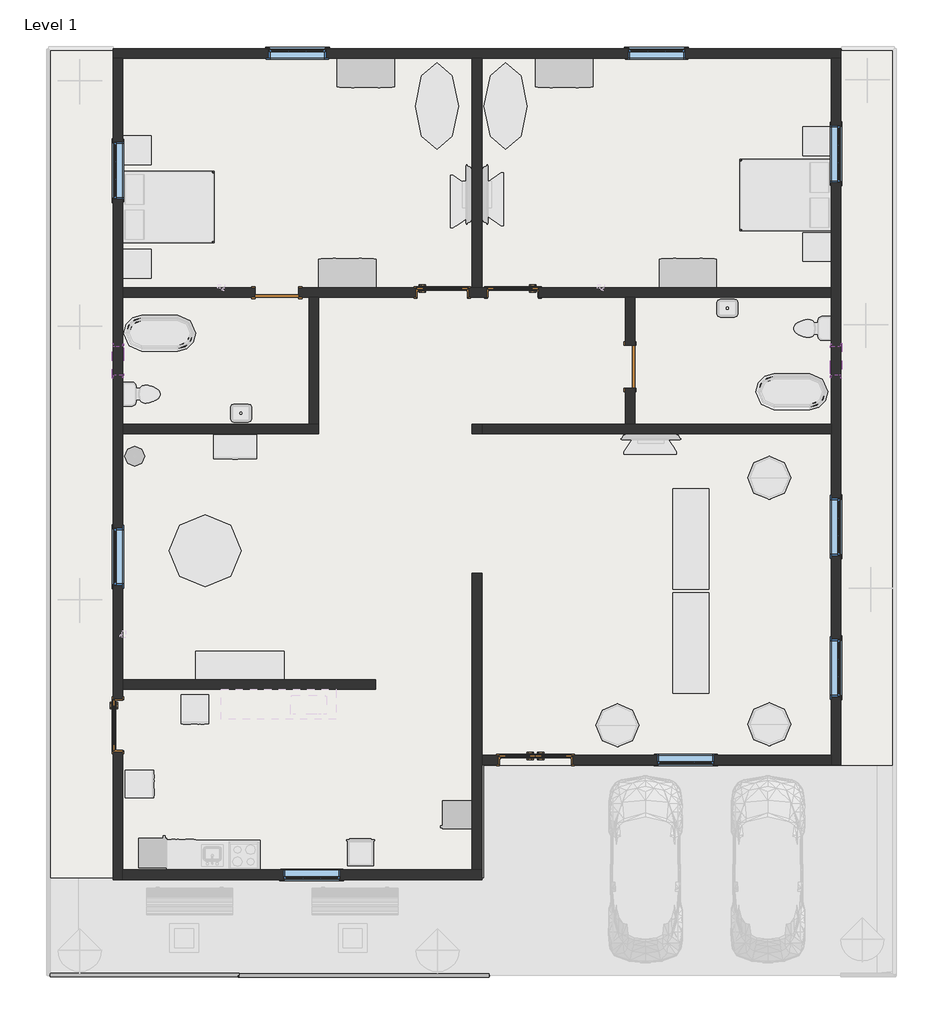
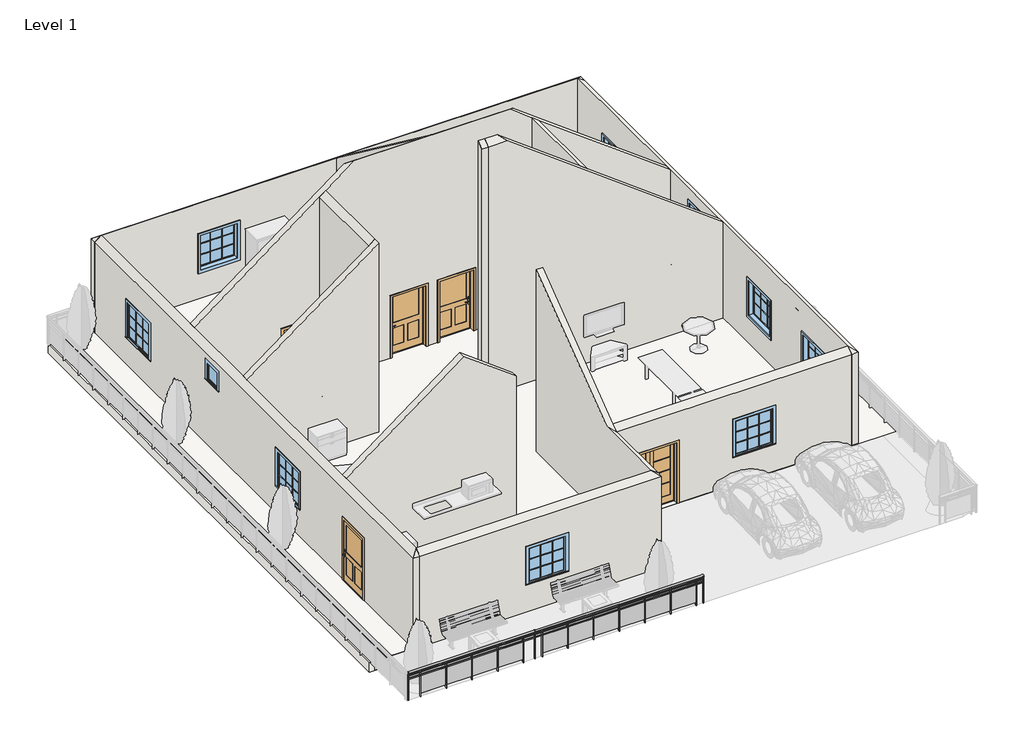
# One storey, part 1 of 3: 14 walls, 11 windows, 6 doors, 2 railings, 1 slab.
"""IFC4 building model written with IfcOpenShell, lengths in millimetres."""

from ifc_helpers import new_model, si_unit, point, frame, origin, origin_with_axes, place, context, project, spatial, polyline, ellipse_curve, trimmed, outline, extrude, faceted_brep, transform, mapped, element, save
from ifc_brep_helpers import plane_surface, extruded_surface, advanced_brep
from components import door_e0076512, door_374e07cf, door_b03bd389, door_719f80de, door_54dd4da4, window_7418cbd4, window_e41d21a6

model = new_model("IFC4")

# Units and contexts
model_context = context("Model", 3, world=origin())
ifc_project = project(units=[si_unit("LENGTHUNIT", "METRE", prefix="MILLI")], contexts=[model_context])

# Site, building, storey
site = spatial("IfcSite", under=ifc_project)
building = spatial("IfcBuilding", under=site)
storey = spatial("IfcBuildingStorey", under=building, Name="Level 1", Elevation=0.0)

# Doors
placement = place(None, origin())
door_shape = door_e0076512(model_context)
element("IfcDoor", 1, ObjectType="42\" x 80\"", at=placement, inside=storey, context=model_context, shape_type="MappedRepresentation", body=[
    mapped(door_shape, transform((-8583.7892853, 8379.5299175, 0.0), x_axis=(1.0, 0.0, 0.0), y_axis=(0.0, 1.0, 0.0), z_axis=(0.0, 0.0, 1.0))),
])
door_2_shape = door_374e07cf(model_context)
element("IfcDoor", 2, ObjectType="42\" x 80\"", at=placement, inside=storey, context=model_context, shape_type="MappedRepresentation", body=[
    mapped(door_2_shape, transform((-10082.3892853, 8379.5299175, 0.0), x_axis=(-1.0, 0.0, 0.0), y_axis=(0.0, -1.0, 0.0), z_axis=(0.0, 0.0, 1.0))),
])
element("IfcDoor", 3, ObjectType="42\" x 80\"", at=placement, inside=storey, context=model_context, shape_type="MappedRepresentation", body=[
    mapped(door_shape, transform((-16981.6642853, -818.4450825, 0.0), x_axis=(0.0, 1.0, 0.0), y_axis=(-1.0, 0.0, 0.0), z_axis=(0.0, 0.0, 1.0))),
])
door_3_shape = door_b03bd389(model_context)
element("IfcDoor", 4, ObjectType="Door-Exterior-Double-Full Glass-Wood_Clad : 60\" x 80\"", at=placement, inside=storey, context=model_context, shape_type="MappedRepresentation", body=[
    mapped(door_3_shape, transform((-8101.1892853, -1551.8700825, 0.0), x_axis=(1.0, 0.0, 0.0), y_axis=(0.0, 1.0, 0.0), z_axis=(0.0, 0.0, 1.0))),
])
door_4_shape = door_719f80de(model_context)
element("IfcDoor", 5, ObjectType="Single-Flush : 36\" x 84\"", at=placement, inside=storey, context=model_context, shape_type="MappedRepresentation", body=[
    mapped(door_4_shape, transform((-13600.2892853, 8376.3549175, 0.0), x_axis=(1.0, 0.0, 0.0), y_axis=(0.0, 1.0, 0.0), z_axis=(0.0, 0.0, 1.0))),
])
door_5_shape = door_54dd4da4(model_context)
element("IfcDoor", 6, ObjectType="Single-Flush : 36\" x 84\"", at=placement, inside=storey, context=model_context, shape_type="MappedRepresentation", body=[
    mapped(door_5_shape, transform((-6094.5892853, 6801.5549175, 0.0), x_axis=(0.0, -1.0, 0.0), y_axis=(1.0, 0.0, 0.0), z_axis=(0.0, 0.0, 1.0))),
])

# Railings
element("IfcRailing", 7, ObjectType="Glass Panel - Bottom Fill", at=placement, inside=storey, context=model_context, shape_type="SolidModel", body=[
    advanced_brep(
    [(-18419.3589891, -6088.9450825, 914.4), (-18419.3589891, -6165.1450825, 914.4), (-14406.1589891, -6088.9450825, 914.4), (-14406.1589891, -6165.1450825, 914.4)],
    [
        (0, 1, ellipse_curve(frame((-18419.3589891, -6127.0450825, 914.4), z_axis=(-1.0, 0.0, 0.0), x_axis=(0.0, -1.0, 0.0)), 38.1, 28.575)),
        (1, 0, ellipse_curve(frame((-18419.3589891, -6127.0450825, 914.4), z_axis=(-1.0, 0.0, 0.0), x_axis=(0.0, -1.0, 0.0)), 38.1, 28.575)),
        (2, 3, ellipse_curve(frame((-14406.1589891, -6127.0450825, 914.4), z_axis=(1.0, 0.0, 0.0), x_axis=(0.0, -1.0, 0.0)), 38.1, 28.575)),
        (3, 2, ellipse_curve(frame((-14406.1589891, -6127.0450825, 914.4), z_axis=(1.0, 0.0, 0.0), x_axis=(0.0, -1.0, 0.0)), 38.1, 28.575)),
        (0, 2),
        (3, 1),
    ],
    [
        plane_surface(frame((-18419.3589891, -6127.0450825, 914.4), z_axis=(-1.0, 0.0, 0.0), x_axis=(0.0, 1.0, 0.0))),
        plane_surface(frame((-14406.1589891, -6127.0450825, 914.4), z_axis=(1.0, 0.0, 0.0), x_axis=(0.0, 1.0, 0.0))),
        extruded_surface(trimmed(ellipse_curve(frame((-14406.1589891, -6127.0450825, 914.4), z_axis=(-1.0, 0.0, 0.0), x_axis=(0.0, -1.0, 0.0)), 38.1, 28.575), [point((-14406.1589891, -6088.9450825, 914.4))], [point((-14406.1589891, -6165.1450825, 914.4))], True, "CARTESIAN"), (-4013.2000000000007, 0.0, 0.0), 4013.2000000000007),
        extruded_surface(trimmed(ellipse_curve(frame((-14406.1589891, -6127.0450825, 914.4), z_axis=(-1.0, 0.0, 0.0), x_axis=(0.0, -1.0, 0.0)), 38.1, 28.575), [point((-14406.1589891, -6165.1450825, 914.4))], [point((-14406.1589891, -6088.9450825, 914.4))], True, "CARTESIAN"), (-4013.2000000000007, 0.0, 0.0), 4013.2000000000007),
    ],
    [
        (0, [[1, 2]]),
        (1, [[3, 4]]),
        (2, [[-1, 5, -4, 6]]),
        (3, [[-2, -6, -3, -5]]),
    ],
),
    extrude(outline(polyline([(-18419.3589891, -6139.7450825), (-18419.3589891, -6114.3450825), (-14406.1589891, -6114.3450825), (-14406.1589891, -6139.7450825), (-18419.3589891, -6139.7450825)])), frame((0.0, 0.0, 800.1), z_axis=(0.0, 0.0, 1.0), x_axis=(1.0, 0.0, 0.0)), (0.0, 0.0, 1.0), 25.4),
    extrude(outline(polyline([(-18419.3589891, -6139.7450825), (-18419.3589891, -6114.3450825), (-14406.1589891, -6114.3450825), (-14406.1589891, -6139.7450825), (-18419.3589891, -6139.7450825)])), frame((0.0, 0.0, 698.5), z_axis=(0.0, 0.0, 1.0), x_axis=(1.0, 0.0, 0.0)), (0.0, 0.0, 1.0), 25.4),
    extrude(outline(polyline([(-14793.5089891, -6152.4450825), (-14793.5089891, -6101.6450825), (-14780.8089891, -6101.6450825), (-14780.8089891, -6152.4450825), (-14793.5089891, -6152.4450825)])), origin_with_axes(), (0.0, 0.0, 1.0), 885.6788223),
    extrude(outline(polyline([(-15599.9589891, -6120.5099255), (-14787.1589891, -6120.5099255), (-14787.1589891, -6126.8599255), (-15599.9589891, -6126.8599255), (-15599.9589891, -6120.5099255)])), frame((0.0, 0.0, 101.6), z_axis=(0.0, 0.0, 1.0), x_axis=(1.0, 0.0, 0.0)), (0.0, 0.0, 1.0), 596.9),
    extrude(outline(polyline([(-15606.3089891, -6152.4450825), (-15606.3089891, -6101.6450825), (-15593.6089891, -6101.6450825), (-15593.6089891, -6152.4450825), (-15606.3089891, -6152.4450825)])), origin_with_axes(), (0.0, 0.0, 1.0), 885.6788223),
    extrude(outline(polyline([(-16412.7589891, -6120.5099255), (-15599.9589891, -6120.5099255), (-15599.9589891, -6126.8599255), (-16412.7589891, -6126.8599255), (-16412.7589891, -6120.5099255)])), frame((0.0, 0.0, 101.6), z_axis=(0.0, 0.0, 1.0), x_axis=(1.0, 0.0, 0.0)), (0.0, 0.0, 1.0), 596.9),
    extrude(outline(polyline([(-16419.1089891, -6152.4450825), (-16419.1089891, -6101.6450825), (-16406.4089891, -6101.6450825), (-16406.4089891, -6152.4450825), (-16419.1089891, -6152.4450825)])), origin_with_axes(), (0.0, 0.0, 1.0), 885.6788223),
    extrude(outline(polyline([(-17225.5589891, -6120.5099255), (-16412.7589891, -6120.5099255), (-16412.7589891, -6126.8599255), (-17225.5589891, -6126.8599255), (-17225.5589891, -6120.5099255)])), frame((0.0, 0.0, 101.6), z_axis=(0.0, 0.0, 1.0), x_axis=(1.0, 0.0, 0.0)), (0.0, 0.0, 1.0), 596.9),
    extrude(outline(polyline([(-17231.9089891, -6152.4450825), (-17231.9089891, -6101.6450825), (-17219.2089891, -6101.6450825), (-17219.2089891, -6152.4450825), (-17231.9089891, -6152.4450825)])), origin_with_axes(), (0.0, 0.0, 1.0), 885.6788223),
    extrude(outline(polyline([(-18038.3589891, -6120.5099255), (-17225.5589891, -6120.5099255), (-17225.5589891, -6126.8599255), (-18038.3589891, -6126.8599255), (-18038.3589891, -6120.5099255)])), frame((0.0, 0.0, 101.6), z_axis=(0.0, 0.0, 1.0), x_axis=(1.0, 0.0, 0.0)), (0.0, 0.0, 1.0), 596.9),
    extrude(outline(polyline([(-18044.7089891, -6152.4450825), (-18044.7089891, -6101.6450825), (-18032.0089891, -6101.6450825), (-18032.0089891, -6152.4450825), (-18044.7089891, -6152.4450825)])), origin_with_axes(), (0.0, 0.0, 1.0), 885.6788223),
    extrude(outline(polyline([(-14418.8589891, -6136.5700825), (-14418.8589891, -6117.5200825), (-14399.8089891, -6117.5200825), (-14399.8089891, -6136.5700825), (-14418.8589891, -6136.5700825)])), origin_with_axes(), (0.0, 0.0, 1.0), 885.6788223),
    extrude(outline(polyline([(-18425.7089891, -6136.5700825), (-18425.7089891, -6117.5200825), (-18406.6589891, -6117.5200825), (-18406.6589891, -6136.5700825), (-18425.7089891, -6136.5700825)])), origin_with_axes(), (0.0, 0.0, 1.0), 885.6788223),
])
element("IfcRailing", 8, ObjectType="Glass Panel - Bottom Fill", at=placement, inside=storey, context=model_context, shape_type="SolidModel", body=[
    advanced_brep(
    [(-14425.2089891, -6098.4700825, 914.4), (-14425.2089891, -6174.6700825, 914.4), (-9091.2089891, -6098.4700825, 914.4), (-9091.2089891, -6174.6700825, 914.4)],
    [
        (0, 1, ellipse_curve(frame((-14425.2089891, -6136.5700825, 914.4), z_axis=(-1.0, 0.0, 0.0), x_axis=(0.0, -1.0, 0.0)), 38.1, 28.575)),
        (1, 0, ellipse_curve(frame((-14425.2089891, -6136.5700825, 914.4), z_axis=(-1.0, 0.0, 0.0), x_axis=(0.0, -1.0, 0.0)), 38.1, 28.575)),
        (2, 3, ellipse_curve(frame((-9091.2089891, -6136.5700825, 914.4), z_axis=(1.0, 0.0, 0.0), x_axis=(0.0, -1.0, 0.0)), 38.1, 28.575)),
        (3, 2, ellipse_curve(frame((-9091.2089891, -6136.5700825, 914.4), z_axis=(1.0, 0.0, 0.0), x_axis=(0.0, -1.0, 0.0)), 38.1, 28.575)),
        (0, 2),
        (3, 1),
    ],
    [
        plane_surface(frame((-14425.2089891, -6136.5700825, 914.4), z_axis=(-1.0, 0.0, 0.0), x_axis=(0.0, 1.0, 0.0))),
        plane_surface(frame((-9091.2089891, -6136.5700825, 914.4), z_axis=(1.0, 0.0, 0.0), x_axis=(0.0, 1.0, 0.0))),
        extruded_surface(trimmed(ellipse_curve(frame((-9091.2089891, -6136.5700825, 914.4), z_axis=(-1.0, 0.0, 0.0), x_axis=(0.0, -1.0, 0.0)), 38.1, 28.575), [point((-9091.2089891, -6098.4700825, 914.4))], [point((-9091.2089891, -6174.6700825, 914.4))], True, "CARTESIAN"), (-5334.0, 0.0, 0.0), 5334.0),
        extruded_surface(trimmed(ellipse_curve(frame((-9091.2089891, -6136.5700825, 914.4), z_axis=(-1.0, 0.0, 0.0), x_axis=(0.0, -1.0, 0.0)), 38.1, 28.575), [point((-9091.2089891, -6174.6700825, 914.4))], [point((-9091.2089891, -6098.4700825, 914.4))], True, "CARTESIAN"), (-5334.0, 0.0, 0.0), 5334.0),
    ],
    [
        (0, [[1, 2]]),
        (1, [[3, 4]]),
        (2, [[-1, 5, -4, 6]]),
        (3, [[-2, -6, -3, -5]]),
    ],
),
    extrude(outline(polyline([(-14425.2089891, -6149.2700825), (-14425.2089891, -6123.8700825), (-9091.2089891, -6123.8700825), (-9091.2089891, -6149.2700825), (-14425.2089891, -6149.2700825)])), frame((0.0, 0.0, 800.1), z_axis=(0.0, 0.0, 1.0), x_axis=(1.0, 0.0, 0.0)), (0.0, 0.0, 1.0), 25.4),
    extrude(outline(polyline([(-14425.2089891, -6149.2700825), (-14425.2089891, -6123.8700825), (-9091.2089891, -6123.8700825), (-9091.2089891, -6149.2700825), (-14425.2089891, -6149.2700825)])), frame((0.0, 0.0, 698.5), z_axis=(0.0, 0.0, 1.0), x_axis=(1.0, 0.0, 0.0)), (0.0, 0.0, 1.0), 25.4),
    extrude(outline(polyline([(-9326.1589891, -6161.9700825), (-9326.1589891, -6111.1700825), (-9313.4589891, -6111.1700825), (-9313.4589891, -6161.9700825), (-9326.1589891, -6161.9700825)])), origin_with_axes(), (0.0, 0.0, 1.0), 885.6788223),
    extrude(outline(polyline([(-10132.6089891, -6130.0349255), (-9319.8089891, -6130.0349255), (-9319.8089891, -6136.3849255), (-10132.6089891, -6136.3849255), (-10132.6089891, -6130.0349255)])), frame((0.0, 0.0, 101.6), z_axis=(0.0, 0.0, 1.0), x_axis=(1.0, 0.0, 0.0)), (0.0, 0.0, 1.0), 596.9),
    extrude(outline(polyline([(-10138.9589891, -6161.9700825), (-10138.9589891, -6111.1700825), (-10126.2589891, -6111.1700825), (-10126.2589891, -6161.9700825), (-10138.9589891, -6161.9700825)])), origin_with_axes(), (0.0, 0.0, 1.0), 885.6788223),
    extrude(outline(polyline([(-10945.4089891, -6130.0349255), (-10132.6089891, -6130.0349255), (-10132.6089891, -6136.3849255), (-10945.4089891, -6136.3849255), (-10945.4089891, -6130.0349255)])), frame((0.0, 0.0, 101.6), z_axis=(0.0, 0.0, 1.0), x_axis=(1.0, 0.0, 0.0)), (0.0, 0.0, 1.0), 596.9),
    extrude(outline(polyline([(-10951.7589891, -6161.9700825), (-10951.7589891, -6111.1700825), (-10939.0589891, -6111.1700825), (-10939.0589891, -6161.9700825), (-10951.7589891, -6161.9700825)])), origin_with_axes(), (0.0, 0.0, 1.0), 885.6788223),
    extrude(outline(polyline([(-11758.2089891, -6130.0349255), (-10945.4089891, -6130.0349255), (-10945.4089891, -6136.3849255), (-11758.2089891, -6136.3849255), (-11758.2089891, -6130.0349255)])), frame((0.0, 0.0, 101.6), z_axis=(0.0, 0.0, 1.0), x_axis=(1.0, 0.0, 0.0)), (0.0, 0.0, 1.0), 596.9),
    extrude(outline(polyline([(-11764.5589891, -6161.9700825), (-11764.5589891, -6111.1700825), (-11751.8589891, -6111.1700825), (-11751.8589891, -6161.9700825), (-11764.5589891, -6161.9700825)])), origin_with_axes(), (0.0, 0.0, 1.0), 885.6788223),
    extrude(outline(polyline([(-12571.0089891, -6130.0349255), (-11758.2089891, -6130.0349255), (-11758.2089891, -6136.3849255), (-12571.0089891, -6136.3849255), (-12571.0089891, -6130.0349255)])), frame((0.0, 0.0, 101.6), z_axis=(0.0, 0.0, 1.0), x_axis=(1.0, 0.0, 0.0)), (0.0, 0.0, 1.0), 596.9),
    extrude(outline(polyline([(-12577.3589891, -6161.9700825), (-12577.3589891, -6111.1700825), (-12564.6589891, -6111.1700825), (-12564.6589891, -6161.9700825), (-12577.3589891, -6161.9700825)])), origin_with_axes(), (0.0, 0.0, 1.0), 885.6788223),
    extrude(outline(polyline([(-13383.8089891, -6130.0349255), (-12571.0089891, -6130.0349255), (-12571.0089891, -6136.3849255), (-13383.8089891, -6136.3849255), (-13383.8089891, -6130.0349255)])), frame((0.0, 0.0, 101.6), z_axis=(0.0, 0.0, 1.0), x_axis=(1.0, 0.0, 0.0)), (0.0, 0.0, 1.0), 596.9),
    extrude(outline(polyline([(-13390.1589891, -6161.9700825), (-13390.1589891, -6111.1700825), (-13377.4589891, -6111.1700825), (-13377.4589891, -6161.9700825), (-13390.1589891, -6161.9700825)])), origin_with_axes(), (0.0, 0.0, 1.0), 885.6788223),
    extrude(outline(polyline([(-14196.6089891, -6130.0349255), (-13383.8089891, -6130.0349255), (-13383.8089891, -6136.3849255), (-14196.6089891, -6136.3849255), (-14196.6089891, -6130.0349255)])), frame((0.0, 0.0, 101.6), z_axis=(0.0, 0.0, 1.0), x_axis=(1.0, 0.0, 0.0)), (0.0, 0.0, 1.0), 596.9),
    extrude(outline(polyline([(-14202.9589891, -6161.9700825), (-14202.9589891, -6111.1700825), (-14190.2589891, -6111.1700825), (-14190.2589891, -6161.9700825), (-14202.9589891, -6161.9700825)])), origin_with_axes(), (0.0, 0.0, 1.0), 885.6788223),
    extrude(outline(polyline([(-9103.9089891, -6146.0950825), (-9103.9089891, -6127.0450825), (-9084.8589891, -6127.0450825), (-9084.8589891, -6146.0950825), (-9103.9089891, -6146.0950825)])), origin_with_axes(), (0.0, 0.0, 1.0), 885.6788223),
    extrude(outline(polyline([(-14431.5589891, -6146.0950825), (-14431.5589891, -6127.0450825), (-14412.5089891, -6127.0450825), (-14412.5089891, -6146.0950825), (-14431.5589891, -6146.0950825)])), origin_with_axes(), (0.0, 0.0, 1.0), 885.6788223),
])

# Slab
element("IfcSlab", 9, ObjectType="Generic - 12\"", at=placement, inside=storey, context=model_context, shape_type="SweptSolid", body=[
    extrude(outline(polyline([(-429.8089891, 13545.2549175), (-429.8089891, -1669.3450825), (-9206.0892853, -1669.3450825), (-9206.0892853, -4056.9450825), (-18451.6892853, -4056.9450825), (-18451.6892853, 13545.2549175), (-429.8089891, 13545.2549175)])), frame((0.0, 0.0, -304.8), z_axis=(0.0, 0.0, 1.0), x_axis=(1.0, 0.0, 0.0)), (0.0, 0.0, 1.0), 304.8),
])

# Walls
element("IfcWall", 10, ObjectType="Generic - 8\"", at=placement, inside=storey, context=model_context, shape_type="Brep", body=[
    faceted_brep([(-17080.0892853, 13354.7549175, 0.0), (-16876.8892853, 13354.7549175, 0.0), (-9447.3892853, 13354.7549175, 0.0), (-9244.1892853, 13354.7549175, 0.0), (-1814.6892853, 13354.7549175, 0.0), (-1611.4892853, 13354.7549175, 0.0), (-1611.4892853, 13354.7549175, 3048.0), (-1801.9892853, 13354.7549175, 3190.875), (-1814.6892853, 13354.7549175, 3190.875), (-9244.1892853, 13354.7549175, 3190.875), (-9447.3892853, 13354.7549175, 3190.875), (-16876.8892853, 13354.7549175, 3190.875), (-16889.5892853, 13354.7549175, 3190.875), (-17080.0892853, 13354.7549175, 3048.0), (-12552.5392853, 13354.7549175, 2133.6), (-12552.5392853, 13354.7549175, 914.4), (-13771.7392853, 13354.7549175, 914.4), (-13771.7392853, 13354.7549175, 2133.6), (-4919.8392853, 13354.7549175, 2133.6), (-4919.8392853, 13354.7549175, 914.4), (-6139.0392853, 13354.7549175, 914.4), (-6139.0392853, 13354.7549175, 2133.6), (-17080.0892853, 13557.9549175, 0.0), (-17080.0892853, 13557.9549175, 3048.0), (-1611.4892853, 13557.9549175, 3048.0), (-1611.4892853, 13557.9549175, 0.0), (-12552.5392853, 13557.9549175, 2133.6), (-13771.7392853, 13557.9549175, 2133.6), (-13771.7392853, 13557.9549175, 914.4), (-12552.5392853, 13557.9549175, 914.4), (-4919.8392853, 13557.9549175, 2133.6), (-6139.0392853, 13557.9549175, 2133.6), (-6139.0392853, 13557.9549175, 914.4), (-4919.8392853, 13557.9549175, 914.4), (-1611.4892853, 13545.2549175, 3048.0), (-17080.0892853, 13545.2549175, 3048.0)], [[[0, 1, 2, 3, 4, 5, 6, 7, 8, 9, 10, 11, 12, 13], [14, 15, 16, 17], [18, 19, 20, 21]], [[22, 23, 24, 25], [26, 27, 28, 29], [30, 31, 32, 33]], [[5, 4, 3, 2, 1, 0, 22, 25]], [[6, 5, 25, 24, 34]], [[0, 13, 35, 23, 22]], [[15, 14, 26, 29]], [[16, 15, 29, 28]], [[17, 16, 28, 27]], [[14, 17, 27, 26]], [[19, 18, 30, 33]], [[20, 19, 33, 32]], [[21, 20, 32, 31]], [[18, 21, 31, 30]], [[34, 24, 23, 35]], [[13, 12, 35]], [[12, 11, 10, 9, 8, 7, 34, 35]], [[7, 6, 34]]]),
])
element("IfcWall", 11, ObjectType="Generic - 8\"", at=placement, inside=storey, context=model_context, shape_type="Brep", body=[
    faceted_brep([(-1814.6892853, 13354.7549175, 0.0), (-1814.6892853, 8477.9549175, 0.0), (-1814.6892853, 8274.7549175, 0.0), (-1814.6892853, 5582.3549175, 0.0), (-1814.6892853, 5379.1549175, 0.0), (-1814.6892853, -1453.4450825, 0.0), (-1814.6892853, -1656.6450825, 0.0), (-1814.6892853, -1656.6450825, 3048.0), (-1814.6892853, -1453.4450825, 3200.4), (-1814.6892853, 5379.1549175, 3200.4), (-1814.6892853, 5582.3549175, 3200.4), (-1814.6892853, 8274.7549175, 3200.4), (-1814.6892853, 8477.9549175, 3200.4), (-1814.6892853, 13342.0549175, 3200.4), (-1814.6892853, 13354.7549175, 3190.875), (-1814.6892853, 10713.1549175, 2133.6), (-1814.6892853, 10713.1549175, 914.4), (-1814.6892853, 11932.3549175, 914.4), (-1814.6892853, 11932.3549175, 2133.6), (-1814.6892853, 2788.3549175, 2133.6), (-1814.6892853, 2788.3549175, 914.4), (-1814.6892853, 4007.5549175, 914.4), (-1814.6892853, 4007.5549175, 2133.6), (-1814.6892853, -208.8450825, 2133.6), (-1814.6892853, -208.8450825, 914.4), (-1814.6892853, 1010.3549175, 914.4), (-1814.6892853, 1010.3549175, 2133.6), (-1814.6892853, 6623.7549175, 2768.6), (-1814.6892853, 6623.7549175, 2159.0), (-1814.6892853, 7233.3549175, 2159.0), (-1814.6892853, 7233.3549175, 2768.6), (-1611.4892853, 13354.7549175, 0.0), (-1611.4892853, 13354.7549175, 3048.0), (-1611.4892853, -1656.6450825, 3048.0), (-1611.4892853, -1656.6450825, 0.0), (-1611.4892853, 10713.1549175, 2133.6), (-1611.4892853, 11932.3549175, 2133.6), (-1611.4892853, 11932.3549175, 914.4), (-1611.4892853, 10713.1549175, 914.4), (-1611.4892853, 2788.3549175, 2133.6), (-1611.4892853, 4007.5549175, 2133.6), (-1611.4892853, 4007.5549175, 914.4), (-1611.4892853, 2788.3549175, 914.4), (-1611.4892853, -208.8450825, 2133.6), (-1611.4892853, 1010.3549175, 2133.6), (-1611.4892853, 1010.3549175, 914.4), (-1611.4892853, -208.8450825, 914.4), (-1611.4892853, 6623.7549175, 2768.6), (-1611.4892853, 7233.3549175, 2768.6), (-1611.4892853, 7233.3549175, 2159.0), (-1611.4892853, 6623.7549175, 2159.0), (-1801.9892853, 13354.7549175, 3190.875)], [[[0, 1, 2, 3, 4, 5, 6, 7, 8, 9, 10, 11, 12, 13, 14], [15, 16, 17, 18], [19, 20, 21, 22], [23, 24, 25, 26], [27, 28, 29, 30]], [[31, 32, 33, 34], [35, 36, 37, 38], [39, 40, 41, 42], [43, 44, 45, 46], [47, 48, 49, 50]], [[6, 5, 4, 3, 2, 1, 0, 31, 34]], [[0, 14, 51, 32, 31]], [[7, 6, 34, 33]], [[16, 15, 35, 38]], [[17, 16, 38, 37]], [[18, 17, 37, 36]], [[15, 18, 36, 35]], [[20, 19, 39, 42]], [[21, 20, 42, 41]], [[22, 21, 41, 40]], [[19, 22, 40, 39]], [[24, 23, 43, 46]], [[25, 24, 46, 45]], [[26, 25, 45, 44]], [[23, 26, 44, 43]], [[28, 27, 47, 50]], [[29, 28, 50, 49]], [[30, 29, 49, 48]], [[27, 30, 48, 47]], [[14, 13, 51]], [[13, 12, 11, 10, 9, 8, 33, 32, 51]], [[8, 7, 33]]]),
])
element("IfcWall", 12, ObjectType="Generic - 8\"", at=placement, inside=storey, context=model_context, shape_type="Brep", body=[
    faceted_brep([(-1814.6892853, -1453.4450825, 3200.4), (-1814.6892853, -1453.4450825, 0.0), (-7313.7892853, -1453.4450825, 0.0), (-7313.7892853, -1453.4450825, 2057.4), (-8888.5892853, -1453.4450825, 2057.4), (-8888.5892853, -1453.4450825, 0.0), (-9244.1892853, -1453.4450825, 0.0), (-9244.1892853, -1453.4450825, 3200.4), (-5516.7392853, -1453.4450825, 2133.6), (-5516.7392853, -1453.4450825, 914.4), (-4297.5392853, -1453.4450825, 914.4), (-4297.5392853, -1453.4450825, 2133.6), (-1814.6892853, -1656.6450825, 0.0), (-1814.6892853, -1656.6450825, 3048.0), (-9244.1892853, -1656.6450825, 3048.0), (-9244.1892853, -1656.6450825, 0.0), (-8888.5892853, -1656.6450825, 0.0), (-8888.5892853, -1656.6450825, 2057.4), (-7313.7892853, -1656.6450825, 2057.4), (-7313.7892853, -1656.6450825, 0.0), (-5516.7392853, -1656.6450825, 2133.6), (-4297.5392853, -1656.6450825, 2133.6), (-4297.5392853, -1656.6450825, 914.4), (-5516.7392853, -1656.6450825, 914.4)], [[[0, 1, 2, 3, 4, 5, 6, 7], [8, 9, 10, 11]], [[12, 13, 14, 15, 16, 17, 18, 19], [20, 21, 22, 23]], [[1, 12, 19, 2]], [[15, 6, 5, 16]], [[1, 0, 13, 12]], [[7, 6, 15, 14]], [[18, 3, 2, 19]], [[3, 18, 17, 4]], [[4, 17, 16, 5]], [[9, 8, 20, 23]], [[10, 9, 23, 22]], [[11, 10, 22, 21]], [[8, 11, 21, 20]], [[0, 7, 14, 13]]]),
])
element("IfcWall", 13, ObjectType="Generic - 8\"", at=placement, inside=storey, context=model_context, shape_type="Brep", body=[
    faceted_brep([(-17080.0892853, 13354.7549175, 3048.0), (-17080.0892853, 13354.7549175, 0.0), (-17080.0892853, -259.6450825, 0.0), (-17080.0892853, -259.6450825, 2057.4), (-17080.0892853, -1377.2450825, 2057.4), (-17080.0892853, -1377.2450825, 0.0), (-17080.0892853, -4095.0450825, 0.0), (-17080.0892853, -4095.0450825, 3048.0), (-17080.0892853, 3372.5549175, 2133.6), (-17080.0892853, 2153.3549175, 2133.6), (-17080.0892853, 2153.3549175, 914.4), (-17080.0892853, 3372.5549175, 914.4), (-17080.0892853, 11576.7549175, 2133.6), (-17080.0892853, 10357.5549175, 2133.6), (-17080.0892853, 10357.5549175, 914.4), (-17080.0892853, 11576.7549175, 914.4), (-17080.0892853, 7233.3549175, 2768.6), (-17080.0892853, 6623.7549175, 2768.6), (-17080.0892853, 6623.7549175, 2159.0), (-17080.0892853, 7233.3549175, 2159.0), (-16876.8892853, 13354.7549175, 0.0), (-16876.8892853, 13354.7549175, 3190.875), (-16876.8892853, 13342.0549175, 3200.4), (-16876.8892853, 8477.9549175, 3200.4), (-16876.8892853, 8274.7549175, 3200.4), (-16876.8892853, 5582.3549175, 3200.4), (-16876.8892853, 5379.1549175, 3200.4), (-16876.8892853, 146.7549175, 3200.4), (-16876.8892853, -56.4450825, 3200.4), (-16876.8892853, -3891.8450825, 3200.4), (-16876.8892853, -4095.0450825, 3048.0), (-16876.8892853, -4095.0450825, 0.0), (-16876.8892853, -3891.8450825, 0.0), (-16876.8892853, -1377.2450825, 0.0), (-16876.8892853, -1377.2450825, 2057.4), (-16876.8892853, -259.6450825, 2057.4), (-16876.8892853, -259.6450825, 0.0), (-16876.8892853, -56.4450825, 0.0), (-16876.8892853, 146.7549175, 0.0), (-16876.8892853, 5379.1549175, 0.0), (-16876.8892853, 5582.3549175, 0.0), (-16876.8892853, 8274.7549175, 0.0), (-16876.8892853, 8477.9549175, 0.0), (-16876.8892853, 3372.5549175, 2133.6), (-16876.8892853, 3372.5549175, 914.4), (-16876.8892853, 2153.3549175, 914.4), (-16876.8892853, 2153.3549175, 2133.6), (-16876.8892853, 11576.7549175, 2133.6), (-16876.8892853, 11576.7549175, 914.4), (-16876.8892853, 10357.5549175, 914.4), (-16876.8892853, 10357.5549175, 2133.6), (-16876.8892853, 7233.3549175, 2768.6), (-16876.8892853, 7233.3549175, 2159.0), (-16876.8892853, 6623.7549175, 2159.0), (-16876.8892853, 6623.7549175, 2768.6), (-16889.5892853, 13354.7549175, 3190.875)], [[[0, 1, 2, 3, 4, 5, 6, 7], [8, 9, 10, 11], [12, 13, 14, 15], [16, 17, 18, 19]], [[20, 21, 22, 23, 24, 25, 26, 27, 28, 29, 30, 31, 32, 33, 34, 35, 36, 37, 38, 39, 40, 41, 42], [43, 44, 45, 46], [47, 48, 49, 50], [51, 52, 53, 54]], [[1, 20, 42, 41, 40, 39, 38, 37, 36, 2]], [[31, 6, 5, 33, 32]], [[1, 0, 55, 21, 20]], [[7, 6, 31, 30]], [[35, 3, 2, 36]], [[3, 35, 34, 4]], [[4, 34, 33, 5]], [[44, 43, 8, 11]], [[45, 44, 11, 10]], [[46, 45, 10, 9]], [[43, 46, 9, 8]], [[48, 47, 12, 15]], [[49, 48, 15, 14]], [[50, 49, 14, 13]], [[47, 50, 13, 12]], [[52, 51, 16, 19]], [[53, 52, 19, 18]], [[54, 53, 18, 17]], [[51, 54, 17, 16]], [[0, 7, 29, 28, 27, 26, 25, 24, 23, 22, 55]], [[7, 30, 29]], [[22, 21, 55]]]),
])
element("IfcWall", 14, ObjectType="Generic - 8\"", at=placement, inside=storey, context=model_context, shape_type="Brep", body=[
    faceted_brep([(-16876.8892853, -4095.0450825, 0.0), (-9244.1892853, -4095.0450825, 0.0), (-9244.1892853, -4095.0450825, 3048.0), (-16876.8892853, -4095.0450825, 3048.0), (-13466.9392853, -4095.0450825, 2133.6), (-12247.7392853, -4095.0450825, 2133.6), (-12247.7392853, -4095.0450825, 914.4), (-13466.9392853, -4095.0450825, 914.4), (-16876.8892853, -3891.8450825, 0.0), (-16876.8892853, -3891.8450825, 3200.4), (-9447.3892853, -3891.8450825, 3200.4), (-9244.1892853, -3891.8450825, 3048.0), (-9244.1892853, -3891.8450825, 0.0), (-9447.3892853, -3891.8450825, 0.0), (-13466.9392853, -3891.8450825, 2133.6), (-13466.9392853, -3891.8450825, 914.4), (-12247.7392853, -3891.8450825, 914.4), (-12247.7392853, -3891.8450825, 2133.6)], [[[0, 1, 2, 3], [4, 5, 6, 7]], [[8, 9, 10, 11, 12, 13], [14, 15, 16, 17]], [[1, 0, 8, 13, 12]], [[0, 3, 9, 8]], [[2, 1, 12, 11]], [[15, 14, 4, 7]], [[16, 15, 7, 6]], [[17, 16, 6, 5]], [[14, 17, 5, 4]], [[3, 2, 10, 9]], [[2, 11, 10]]]),
])
element("IfcWall", 15, ObjectType="Generic - 8\"", at=placement, inside=storey, context=model_context, shape_type="SweptSolid", body=[
    extrude(outline(polyline([(13354.7549175, 0.0), (8477.9549175, 0.0), (8477.9549175, 6848.475), (13354.7549175, 3190.875), (13354.7549175, 0.0)])), frame((-9447.3892853, 0.0, 0.0), z_axis=(1.0, 0.0, 0.0), x_axis=(0.0, 1.0, 0.0)), (0.0, 0.0, 1.0), 203.2),
])
element("IfcWall", 16, ObjectType="Generic - 8\"", at=placement, inside=storey, context=model_context, shape_type="SweptSolid", body=[
    extrude(outline(polyline([(0.0, -16876.8892853), (0.0, -11504.7892853), (4743.45, -11504.7892853), (5986.4625, -13162.1392853), (3200.4, -16876.8892853), (0.0, -16876.8892853)])), frame((0.0, -56.4450825, 0.0), z_axis=(0.0, 1.0, 0.0), x_axis=(0.0, 0.0, 1.0)), (0.0, 0.0, 1.0), 203.2),
])
element("IfcWall", 17, ObjectType="Generic - 8\"", at=placement, inside=storey, context=model_context, shape_type="Brep", body=[
    faceted_brep([(-16876.8892853, 5379.1549175, 0.0), (-12711.2892853, 5379.1549175, 0.0), (-12711.2892853, 5379.1549175, 6324.6), (-16876.8892853, 5379.1549175, 3200.4), (-16876.8892853, 5582.3549175, 0.0), (-16876.8892853, 5582.3549175, 3200.4), (-12914.4892853, 5582.3549175, 6172.2), (-12711.2892853, 5582.3549175, 6324.6), (-12711.2892853, 5582.3549175, 0.0), (-12914.4892853, 5582.3549175, 0.0)], [[[0, 1, 2, 3]], [[4, 5, 6, 7, 8, 9]], [[1, 0, 4, 9, 8]], [[0, 3, 5, 4]], [[2, 1, 8, 7]], [[3, 2, 7, 6, 5]]]),
])
element("IfcWall", 18, ObjectType="Generic - 8\"", at=placement, inside=storey, context=model_context, shape_type="SweptSolid", body=[
    extrude(outline(polyline([(6172.2, -12914.4892853), (0.0, -12914.4892853), (0.0, -12711.2892853), (6324.6, -12711.2892853), (6172.2, -12914.4892853)])), frame((0.0, 5582.3549175, 0.0), z_axis=(0.0, 1.0, 0.0), x_axis=(0.0, 0.0, 1.0)), (0.0, 0.0, 1.0), 2692.4),
])
element("IfcWall", 19, ObjectType="Generic - 8\"", at=placement, inside=storey, context=model_context, shape_type="Brep", body=[
    faceted_brep([(-9244.1892853, 5379.1549175, 0.0), (-1814.6892853, 5379.1549175, 0.0), (-1814.6892853, 5379.1549175, 3200.4), (-8647.2892853, 5379.1549175, 8324.85), (-9244.1892853, 5379.1549175, 8324.85), (-9244.1892853, 5582.3549175, 0.0), (-9244.1892853, 5582.3549175, 8477.25), (-8850.4892853, 5582.3549175, 8477.25), (-6196.1892853, 5582.3549175, 6486.525), (-5992.9892853, 5582.3549175, 6334.125), (-1814.6892853, 5582.3549175, 3200.4), (-1814.6892853, 5582.3549175, 0.0), (-5992.9892853, 5582.3549175, 0.0), (-6196.1892853, 5582.3549175, 0.0)], [[[0, 1, 2, 3, 4]], [[5, 6, 7, 8, 9, 10, 11, 12, 13]], [[1, 0, 5, 13, 12, 11]], [[2, 1, 11, 10]], [[0, 4, 6, 5]], [[4, 3, 7, 6]], [[3, 2, 10, 9, 8, 7]]]),
])
element("IfcWall", 20, ObjectType="Generic - 8\"", at=placement, inside=storey, context=model_context, shape_type="Brep", body=[
    faceted_brep([(-6196.1892853, 6344.3549175, 2133.6), (-6196.1892853, 6344.3549175, 0.0), (-6196.1892853, 5582.3549175, 0.0), (-6196.1892853, 5582.3549175, 6486.525), (-6196.1892853, 8274.7549175, 6486.525), (-6196.1892853, 8274.7549175, 0.0), (-6196.1892853, 7258.7549175, 0.0), (-6196.1892853, 7258.7549175, 2133.6), (-5992.9892853, 5582.3549175, 0.0), (-5992.9892853, 6344.3549175, 0.0), (-5992.9892853, 6344.3549175, 2133.6), (-5992.9892853, 7258.7549175, 2133.6), (-5992.9892853, 7258.7549175, 0.0), (-5992.9892853, 8274.7549175, 0.0), (-5992.9892853, 8274.7549175, 6334.125), (-5992.9892853, 5582.3549175, 6334.125)], [[[0, 1, 2, 3, 4, 5, 6, 7]], [[8, 9, 10, 11, 12, 13, 14, 15]], [[6, 5, 13, 12]], [[2, 1, 9, 8]], [[5, 4, 14, 13]], [[3, 2, 8, 15]], [[10, 9, 1, 0]], [[11, 10, 0, 7]], [[12, 11, 7, 6]], [[4, 3, 15, 14]]]),
])
element("IfcWall", 21, ObjectType="Generic - 8\"", at=placement, inside=storey, context=model_context, shape_type="SweptSolid", body=[
    extrude(outline(polyline([(5582.3549175, 0.0), (5379.1549175, 0.0), (5379.1549175, 8324.85), (5582.3549175, 8477.25), (5582.3549175, 0.0)])), frame((-9447.3892853, 0.0, 0.0), z_axis=(1.0, 0.0, 0.0), x_axis=(0.0, 1.0, 0.0)), (0.0, 0.0, 1.0), 203.2),
])
element("IfcWall", 22, ObjectType="Generic - 8\"", at=placement, inside=storey, context=model_context, shape_type="Brep", body=[
    faceted_brep([(-9447.3892853, 2407.3549175, 0.0), (-9447.3892853, -3891.8450825, 0.0), (-9447.3892853, -3891.8450825, 3200.4), (-9447.3892853, -1453.4450825, 3200.4), (-9447.3892853, 2407.3549175, 6096.0), (-9244.1892853, 2407.3549175, 0.0), (-9244.1892853, 2407.3549175, 6096.0), (-9244.1892853, -1453.4450825, 3200.4), (-9244.1892853, -1656.6450825, 3048.0), (-9244.1892853, -3891.8450825, 3048.0), (-9244.1892853, -3891.8450825, 0.0), (-9244.1892853, -1656.6450825, 0.0), (-9244.1892853, -1453.4450825, 0.0)], [[[0, 1, 2, 3, 4]], [[5, 6, 7, 8, 9, 10, 11, 12]], [[1, 0, 5, 12, 11, 10]], [[0, 4, 6, 5]], [[2, 1, 10, 9]], [[4, 3, 8, 7, 6]], [[3, 2, 9, 8]]]),
])
element("IfcWall", 23, ObjectType="INNER WALL", at=placement, inside=storey, context=model_context, shape_type="Brep", body=[
    faceted_brep([(-16876.8892853, 8274.7549175, 3200.4), (-16876.8892853, 8274.7549175, 0.0), (-14057.4892853, 8274.7549175, 0.0), (-14057.4892853, 8274.7549175, 2133.6), (-13143.0892853, 8274.7549175, 2133.6), (-13143.0892853, 8274.7549175, 0.0), (-12914.4892853, 8274.7549175, 0.0), (-12711.2892853, 8274.7549175, 0.0), (-10641.1892853, 8274.7549175, 0.0), (-10641.1892853, 8274.7549175, 2057.4), (-9523.5892853, 8274.7549175, 2057.4), (-9523.5892853, 8274.7549175, 0.0), (-9142.5892853, 8274.7549175, 0.0), (-9142.5892853, 8274.7549175, 2057.4), (-8024.9892853, 8274.7549175, 2057.4), (-8024.9892853, 8274.7549175, 0.0), (-6196.1892853, 8274.7549175, 0.0), (-5992.9892853, 8274.7549175, 0.0), (-1814.6892853, 8274.7549175, 0.0), (-1814.6892853, 8274.7549175, 3200.4), (-5992.9892853, 8274.7549175, 6334.125), (-6196.1892853, 8274.7549175, 6486.525), (-6881.9892853, 8274.7549175, 7000.875), (-11809.5892853, 8274.7549175, 7000.875), (-12711.2892853, 8274.7549175, 6324.6), (-12914.4892853, 8274.7549175, 6172.2), (-16876.8892853, 8477.9549175, 0.0), (-16876.8892853, 8477.9549175, 3200.4), (-12012.7892853, 8477.9549175, 6848.475), (-9447.3892853, 8477.9549175, 6848.475), (-9244.1892853, 8477.9549175, 6848.475), (-6678.7892853, 8477.9549175, 6848.475), (-1814.6892853, 8477.9549175, 3200.4), (-1814.6892853, 8477.9549175, 0.0), (-8024.9892853, 8477.9549175, 0.0), (-8024.9892853, 8477.9549175, 2057.4), (-9142.5892853, 8477.9549175, 2057.4), (-9142.5892853, 8477.9549175, 0.0), (-9244.1892853, 8477.9549175, 0.0), (-9447.3892853, 8477.9549175, 0.0), (-9523.5892853, 8477.9549175, 0.0), (-9523.5892853, 8477.9549175, 2057.4), (-10641.1892853, 8477.9549175, 2057.4), (-10641.1892853, 8477.9549175, 0.0), (-13143.0892853, 8477.9549175, 0.0), (-13143.0892853, 8477.9549175, 2133.6), (-14057.4892853, 8477.9549175, 2133.6), (-14057.4892853, 8477.9549175, 0.0)], [[[0, 1, 2, 3, 4, 5, 6, 7, 8, 9, 10, 11, 12, 13, 14, 15, 16, 17, 18, 19, 20, 21, 22, 23, 24, 25]], [[26, 27, 28, 29, 30, 31, 32, 33, 34, 35, 36, 37, 38, 39, 40, 41, 42, 43, 44, 45, 46, 47]], [[1, 26, 47, 2]], [[33, 18, 17, 16, 15, 34]], [[5, 44, 43, 8, 7, 6]], [[37, 12, 11, 40, 39, 38]], [[1, 0, 27, 26]], [[19, 18, 33, 32]], [[45, 44, 5, 4]], [[46, 45, 4, 3]], [[47, 46, 3, 2]], [[14, 35, 34, 15]], [[35, 14, 13, 36]], [[36, 13, 12, 37]], [[42, 9, 8, 43]], [[9, 42, 41, 10]], [[10, 41, 40, 11]], [[27, 0, 25, 24, 23, 28]], [[23, 22, 31, 30, 29, 28]], [[19, 32, 31, 22, 21, 20]]]),
])

# Windows
window_shape = window_7418cbd4(model_context)
element("IfcWindow", 24, ObjectType="Casement 3x3 with Trim : 48\" x 48\"", at=placement, inside=storey, context=model_context, shape_type="MappedRepresentation", body=[
    mapped(window_shape, transform((-12857.3392853, -3993.4450825, 0.0), x_axis=(-1.0, 0.0, 0.0), y_axis=(0.0, -1.0, 0.0), z_axis=(0.0, 0.0, 1.0))),
])
element("IfcWindow", 25, ObjectType="Casement 3x3 with Trim : 48\" x 48\"", at=placement, inside=storey, context=model_context, shape_type="MappedRepresentation", body=[
    mapped(window_shape, transform((-16978.4892853, 2762.9549175, 0.0), x_axis=(0.0, 1.0, 0.0), y_axis=(-1.0, 0.0, 0.0), z_axis=(0.0, 0.0, 1.0))),
])
element("IfcWindow", 26, ObjectType="Casement 3x3 with Trim : 48\" x 48\"", at=placement, inside=storey, context=model_context, shape_type="MappedRepresentation", body=[
    mapped(window_shape, transform((-16978.4892853, 10967.1549175, 0.0), x_axis=(0.0, 1.0, 0.0), y_axis=(-1.0, 0.0, 0.0), z_axis=(0.0, 0.0, 1.0))),
])
element("IfcWindow", 27, ObjectType="Casement 3x3 with Trim : 48\" x 48\"", at=placement, inside=storey, context=model_context, shape_type="MappedRepresentation", body=[
    mapped(window_shape, transform((-13162.1392853, 13456.3549175, 0.0), x_axis=(1.0, 0.0, 0.0), y_axis=(0.0, 1.0, 0.0), z_axis=(0.0, 0.0, 1.0))),
])
element("IfcWindow", 28, ObjectType="Casement 3x3 with Trim : 48\" x 48\"", at=placement, inside=storey, context=model_context, shape_type="MappedRepresentation", body=[
    mapped(window_shape, transform((-5529.4392853, 13456.3549175, 0.0), x_axis=(1.0, 0.0, 0.0), y_axis=(0.0, 1.0, 0.0), z_axis=(0.0, 0.0, 1.0))),
])
element("IfcWindow", 29, ObjectType="Casement 3x3 with Trim : 48\" x 48\"", at=placement, inside=storey, context=model_context, shape_type="MappedRepresentation", body=[
    mapped(window_shape, transform((-1713.0892853, 11322.7549175, 0.0), x_axis=(0.0, -1.0, 0.0), y_axis=(1.0, 0.0, 0.0), z_axis=(0.0, 0.0, 1.0))),
])
element("IfcWindow", 30, ObjectType="Casement 3x3 with Trim : 48\" x 48\"", at=placement, inside=storey, context=model_context, shape_type="MappedRepresentation", body=[
    mapped(window_shape, transform((-1713.0892853, 3397.9549175, 0.0), x_axis=(0.0, -1.0, 0.0), y_axis=(1.0, 0.0, 0.0), z_axis=(0.0, 0.0, 1.0))),
])
element("IfcWindow", 31, ObjectType="Casement 3x3 with Trim : 48\" x 48\"", at=placement, inside=storey, context=model_context, shape_type="MappedRepresentation", body=[
    mapped(window_shape, transform((-1713.0892853, 400.7549175, 0.0), x_axis=(0.0, -1.0, 0.0), y_axis=(1.0, 0.0, 0.0), z_axis=(0.0, 0.0, 1.0))),
])
element("IfcWindow", 32, ObjectType="Casement 3x3 with Trim : 48\" x 48\"", at=placement, inside=storey, context=model_context, shape_type="MappedRepresentation", body=[
    mapped(window_shape, transform((-4907.1392853, -1555.0450825, 0.0), x_axis=(-1.0, 0.0, 0.0), y_axis=(0.0, -1.0, 0.0), z_axis=(0.0, 0.0, 1.0))),
])
window_2_shape = window_e41d21a6(model_context)
element("IfcWindow", 33, ObjectType="Transom with Trim : 24\" x 24\"", at=placement, inside=storey, context=model_context, shape_type="MappedRepresentation", body=[
    mapped(window_2_shape, transform((-16978.4892853, 6966.6549175, 0.0), x_axis=(0.0, 1.0, 0.0), y_axis=(-1.0, 0.0, 0.0), z_axis=(0.0, 0.0, 1.0))),
])
element("IfcWindow", 34, ObjectType="Transom with Trim : 24\" x 24\"", at=placement, inside=storey, context=model_context, shape_type="MappedRepresentation", body=[
    mapped(window_2_shape, transform((-1713.0892853, 6890.4549175, 0.0), x_axis=(0.0, -1.0, 0.0), y_axis=(1.0, 0.0, 0.0), z_axis=(0.0, 0.0, 1.0))),
])

save(model, "model.ifc")

# Revit data of these elements
# Type "42\" x 80\""
#   Type Mark = "8"
#   Assembly Code = "B2030100"
#   Analytic Construction = "French door, wood frame with single glass"
#   Top Rail = 0' - 4 3/4"
#   Threshold Offset [instance default] = 0' - 0 1/2"
#   Thickness = 0' - 1 3/8"
#   Thermal Resistance (R) = 1.0696 (h·ft²·°F)/BTU
#   Swing Angle [instance default] = 90.00°
#   Stiles = 0' - 4 3/4"
#   Rough Width = 3' - 8"
#   Rough Height = 6' - 9"
#   Lock Rail = 0' - 7 1/8"
#   Height = 6' - 8"
#   Width = 3' - 6"
#   Heat Transfer Coefficient (U) = 0.9350 BTU/(h·ft²·°F)
#   Door Offset [instance default] = 0' - 0"
#   Bottom Rail = 0' - 9 1/2"
#   Threshold [instance default] = yes
#   Function = 1
#   Exterior Trim [instance default] = yes
#   Trim Material = Cherry
#   Threshold Material = Cherry
#   Panel Material = Cherry
#   Glazing = Glass
#   Frame Material = Cherry
#   Door Handle Material = Aluminum
#   Visual Light Transmittance = 0
#   Solar Heat Gain Coefficient = 0
#   Wall Closure = (empty or 0)
#   Construction Type = (empty or 0)
# Type "Door-Exterior-Double-Full Glass-Wood_Clad : 60\" x 80\""
#   Type Mark = "9"
#   Assembly Code = "B2030100"
#   Analytic Construction = "French door, wood frame with double glass"
#   Top Rail = 0' - 4 11/16"
#   Threshold Offset [instance default] = 0' - 0 1/2"
#   Thickness = 0' - 1 3/8"
#   Thermal Resistance (R) = 1.9158 (h·ft²·°F)/BTU
#   Swing Angle [instance default] = 90.00°
#   Stiles = 0' - 4 3/4"
#   Rough Width = 5' - 2"
#   Rough Height = 6' - 9"
#   Panel Width = 2' - 6"
#   Door Offset [instance default] = 0' - 0"
#   Height = 6' - 8"
#   Width = 5' - 0"
#   Heat Transfer Coefficient (U) = 0.5220 BTU/(h·ft²·°F)
#   Bottom Rail = 0' - 9 1/8"
#   Exterior Trim [instance default] = yes
#   Threshold [instance default] = yes
#   Show Grill [instance default] = yes
#   Function = 1
#   Trim Material = Cherry
#   Threshold Material = Cherry
#   Panel Material = Cherry
#   Glazing = Glass
#   Frame Material = Cherry
#   Door Handle Material = Aluminum
#   Visual Light Transmittance = 0
#   Solar Heat Gain Coefficient = 0
#   Wall Closure = (empty or 0)
#   Construction Type = (empty or 0)
# Type "Single-Flush : 36\" x 84\""
#   Type Mark = "1"
#   Construction Type Id = "MDOOR"
#   Assembly Code = "C1020"
#   Analytic Construction = "Metal"
#   Thickness = 0' - 2"
#   Heat Transfer Coefficient (U) = 0.651978 BTU/(h·ft²·°F)
#   Height = 7' - 0"
#   Trim Projection Ext = 0' - 1"
#   Trim Projection Int = 0' - 1"
#   Trim Width = 0' - 3"
#   Width = 3' - 0"
#   Define Thermal Properties by = 1
#   Door Material = Door - Panel
#   Frame Material = Door - Frame
#   Visual Light Transmittance = 0
#   Solar Heat Gain Coefficient = 0
#   Function = (empty or 0)
#   Wall Closure = (empty or 0)
# Type "Glass Panel - Bottom Fill"
#   Assembly Code = "C2010400"
#   built-in parameter 1008612 = 0.0416667 (stored number, unit not read)
#   built-in parameter 1008611 = 0.0416667 (stored number, unit not read)
#   built-in parameter 1008609 = 0.333333 (stored number, unit not read)
#   built-in parameter 1008604 = 0.166667 (stored number, unit not read)
#   built-in parameter 1008603 = 0.166667 (stored number, unit not read)
#   Railing Height = 3' - 0"
#   built-in parameter 1008630 = 2
#   built-in parameter 1008610 = 2
#   built-in parameter 1008618 = Baluster - Square : 3/4"
# Type "Generic - 12\""
#   Assembly Code = "B1010"
#   Function = 0
#   Layers, outside or top first: 1' - 0" no material (function 1)
# Type "Generic - 8\""
#   Assembly Code = "B2010"
#   Layers, outside or top first: 0' - 8" "Brick, Common" (function 1)
# Type "INNER WALL"
#   Assembly Code = "B2010"
#   Layers, outside or top first: 0' - 8" "Brick, Soldier Course" (function 1)
# Type "Casement 3x3 with Trim : 48\" x 48\""
#   Type Mark = "10"
#   Construction Type Id = "GSP4R"
#   Assembly Code = "B2020100"
#   Analytic Construction = "1/8 in Pilkington single glazing"
#   Visual Light Transmittance = 0.9
#   Solar Heat Gain Coefficient = 0.78
#   Heat Transfer Coefficient (U) = 0.6496 BTU/(h·ft²·°F)
#   Height = 4' - 0"
#   Default Sill Height = 3' - 0"
#   Trim Projection - Ext. = 0' - 0 1/2"
#   Trim Projection - Int. = 0' - 0 3/4"
#   Trim Width - Exterior = 0' - 3 1/2"
#   Trim Width - Interior = 0' - 3 1/2"
#   Width = 4' - 0"
#   Window Inset = 0' - 0 3/4"
#   Define Thermal Properties by = 1
#   Glass Pane Material = Glass
#   Sash Material = Sash
#   Trim Exterior Material = Trim
#   Trim Interior Material = Trim
#   Wall Closure = (empty or 0)
# Type "Transom with Trim : 24\" x 24\""
#   Type Mark = "13"
#   Construction Type Id = "GSP4R"
#   Assembly Code = "B2020100"
#   Analytic Construction = "1/8 in Pilkington single glazing"
#   Visual Light Transmittance = 0.9
#   Solar Heat Gain Coefficient = 0.78
#   Heat Transfer Coefficient (U) = 0.6496 BTU/(h·ft²·°F)
#   Height = 2' - 0"
#   Default Sill Height = 7' - 1"
#   Trim Projection - Ext. = 0' - 0 1/2"
#   Trim Projection - Int. = 0' - 0 3/4"
#   Trim Width - Exterior = 0' - 3 1/2"
#   Trim Width - Interior = 0' - 3 1/2"
#   Width = 2' - 0"
#   Window Inset = 0' - 0 3/4"
#   Define Thermal Properties by = 1
#   Glass Pane Material = Glass
#   Sash Material = Sash
#   Trim Exterior Material = Trim
#   Trim Interior Material = Trim
#   Wall Closure = (empty or 0)
# Elements 1, 2, 3 (IfcDoor, "42\" x 80\"")
#   Threshold Offset = 0' - 0 1/2"
#   Swing Angle = 90.00°
#   Door Offset = 0' - 0"
#   Threshold = yes
#   Exterior Trim = yes
#   Phase Created = New Construction
#   Materials on its faces: "Cherry", "Aluminum", "Glass"
# Element 4 (IfcDoor, "Door-Exterior-Double-Full Glass-Wood_Clad : 60\" x 80\"")
#   Threshold Offset = 0' - 0 1/2"
#   Swing Angle = 90.00°
#   Door Offset = 0' - 0"
#   Threshold = yes
#   Show Grill = yes
#   Exterior Trim = yes
#   Phase Created = New Construction
#   Materials on its faces: "Cherry", "Aluminum", "Glass"
# Elements 5, 6 (IfcDoor, "Single-Flush : 36\" x 84\"")
#   Phase Created = New Construction
#   Materials on its faces: "Door - Frame", "Door - Panel"
# Elements 7, 8 (IfcRailing, "Glass Panel - Bottom Fill")
#   Phase Created = New Construction
#   Materials on its faces: "Glass"
# Element 9 (IfcSlab, "Generic - 12\"")
#   Height Offset From Level = 0' - 0"
#   Phase Created = New Construction
#   Materials on its faces: "Default Floor"
# Elements 10, 11, 12, 13, 14, 15, 16, 17, 18, 19, 20, 21, 22 (IfcWall, "Generic - 8\"")
#   Top Offset = 0' - 0"
#   Base Offset = 0' - 0"
#   Unconnected Height = 10' - 0"
#   wall height = 10' - 0"
#   Phase Created = New Construction
#   Base Constraint = Level 1
#   Materials on its faces: "Brick, Common"
# Element 23 (IfcWall, "INNER WALL")
#   Top Offset = 0' - 0"
#   Base Offset = 0' - 0"
#   Unconnected Height = 10' - 0"
#   wall height = 10' - 0"
#   Phase Created = New Construction
#   Base Constraint = Level 1
#   Materials on its faces: "Brick, Soldier Course"
# Element 24 (IfcWindow, "Casement 3x3 with Trim : 48\" x 48\"")
#   Mark = "1"
#   Phase Created = New Construction
#   Materials on its faces: "Sash", "Glass", "Trim"
# Element 25 (IfcWindow, "Casement 3x3 with Trim : 48\" x 48\"")
#   Mark = "2"
#   Phase Created = New Construction
#   Materials on its faces: "Sash", "Glass", "Trim"
# Element 26 (IfcWindow, "Casement 3x3 with Trim : 48\" x 48\"")
#   Mark = "3"
#   Phase Created = New Construction
#   Materials on its faces: "Sash", "Glass", "Trim"
# Element 27 (IfcWindow, "Casement 3x3 with Trim : 48\" x 48\"")
#   Mark = "4"
#   Phase Created = New Construction
#   Materials on its faces: "Sash", "Glass", "Trim"
# Element 28 (IfcWindow, "Casement 3x3 with Trim : 48\" x 48\"")
#   Mark = "5"
#   Phase Created = New Construction
#   Materials on its faces: "Sash", "Glass", "Trim"
# Element 29 (IfcWindow, "Casement 3x3 with Trim : 48\" x 48\"")
#   Mark = "6"
#   Phase Created = New Construction
#   Materials on its faces: "Sash", "Glass", "Trim"
# Element 30 (IfcWindow, "Casement 3x3 with Trim : 48\" x 48\"")
#   Mark = "7"
#   Phase Created = New Construction
#   Materials on its faces: "Sash", "Glass", "Trim"
# Element 31 (IfcWindow, "Casement 3x3 with Trim : 48\" x 48\"")
#   Mark = "8"
#   Phase Created = New Construction
#   Materials on its faces: "Sash", "Glass", "Trim"
# Element 32 (IfcWindow, "Casement 3x3 with Trim : 48\" x 48\"")
#   Mark = "9"
#   Phase Created = New Construction
#   Materials on its faces: "Sash", "Glass", "Trim"
# Element 33 (IfcWindow, "Transom with Trim : 24\" x 24\"")
#   Mark = "10"
#   Phase Created = New Construction
#   Materials on its faces: "Sash", "Trim", "Glass"
# Element 34 (IfcWindow, "Transom with Trim : 24\" x 24\"")
#   Mark = "11"
#   Phase Created = New Construction
#   Materials on its faces: "Sash", "Trim", "Glass"
# Materials
#   "Cherry": class "Wood", colour RGB 226 177 128, transparency 0, Description = "Prunus Serotina", Cost = 0
#   "Glass": class "Glass", colour RGB 0 128 192, transparency 0.75, Description = "Soda Lime Glass", Cost = 0
#   "Aluminum": class "Metal", colour RGB 247 247 247, transparency 0, Description = "Aluminum 6061", Cost = 0
#   "Door - Panel": class "Wood", colour RGB 210 159 95, transparency 0
#   "Door - Frame": colour RGB 118 70 51, transparency 0
#   "Brick, Common": class "Masonry", colour RGB 170 98 104, transparency 0, Description = "Common brick", Cost = 0
#   "Brick, Soldier Course": class "Masonry", colour RGB 170 98 104, transparency 0, Description = "Common brick soldier coursed", Cost = 0
#   "Sash": class "Wood", colour RGB 224 178 126, transparency 0
#   "Trim": class "Wood", colour RGB 224 178 126, transparency 0
#   "Default Floor": colour RGB 128 128 128, transparency 0
# Room at (-12896.744, 10896.195) mm, phase "New Construction", upper level "Level 1", upper offset 10' - 0", lower offset 0' - 0"
#   Number = "1"
#   Name = "M BED ROOM"
# Room at (-5384.126, 10896.195) mm, phase "New Construction", upper level "Level 1", upper offset 10' - 0", lower offset 0' - 0"
#   Number = "2"
#   Name = "M BED ROOM"
# Room at (-14725.544, 6886.652) mm, phase "New Construction", upper level "Level 1", upper offset 10' - 0", lower offset 0' - 0"
#   Number = "3"
#   Name = "TOILET"
# Room at (-3555.326, 6886.652) mm, phase "New Construction", upper level "Level 1", upper offset 10' - 0", lower offset 0' - 0"
#   Number = "4"
#   Name = "TOILET"
# Room at (-13614.241, -1807.726) mm, phase "New Construction", upper level "Level 1", upper offset 10' - 0", lower offset 0' - 0"
#   Number = "5"
#   Name = "KITCHEN AREA"
# Room at (-13614.241, 3088.137) mm, phase "New Construction", upper level "Level 1", upper offset 10' - 0", lower offset 0' - 0"
#   Number = "6"
# Room at (-5384.126, 2412.846) mm, phase "New Construction", upper level "Level 1", upper offset 10' - 0", lower offset 0' - 0"
#   Number = "7"
#   Name = "HALL"
# Room at (-5850.198, -3609.807) mm, phase "New Construction", upper level "Level 1", upper offset 10' - 0", lower offset 0' - 0"
#   Number = "8"
#   Name = "PARKING"
# Room at (-4726.961, -6164.3) mm, phase "New Construction", upper level "Level 1", upper offset 10' - 0", lower offset 0' - 0"
#   Number = "9"
#   Name = "GATE"
# Room at (-17502.503, 3748.513) mm, phase "New Construction", upper level "Level 1", upper offset 10' - 0", lower offset 0' - 0"
#   Number = "10"
#   Name = "VERANDAH"
# Room at (-877.12, 3748.513) mm, phase "New Construction", upper level "Level 1", upper offset 10' - 0", lower offset 0' - 0"
#   Number = "11"
#   Name = "VERANDAH"
